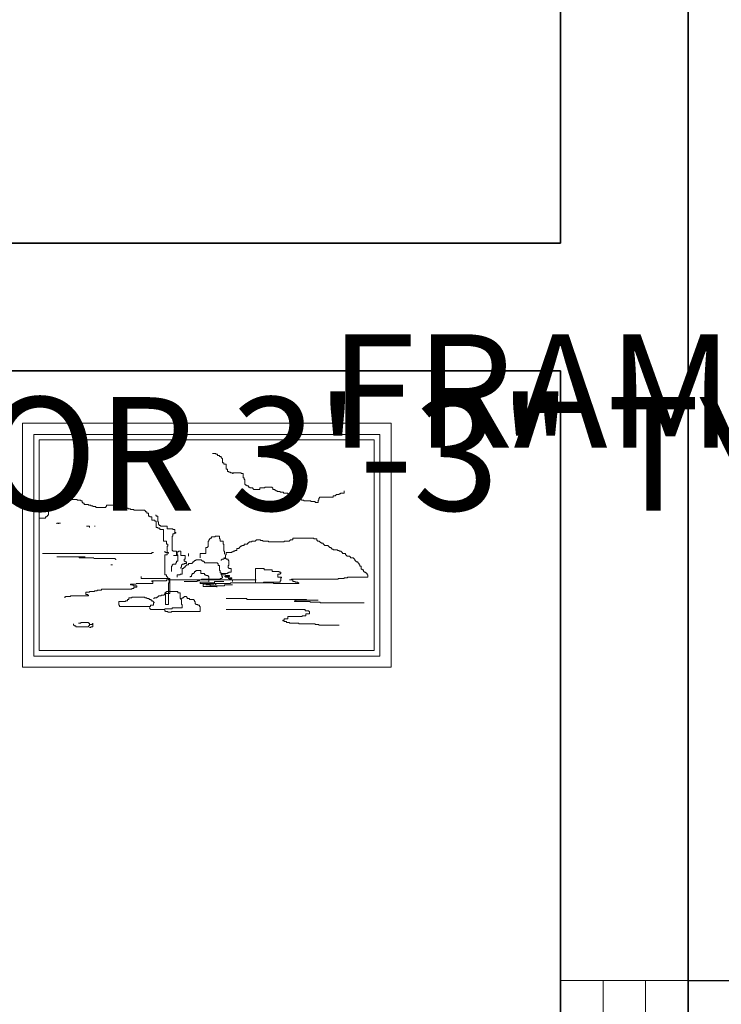
# Model space of a CAD drawing. Units: inches. Extents: x 125 to 976, y 231 to 853.
# Tile 7 of 16: x 418 to 468, y 449 to 519. Entities that reach past the tile are written whole.
import ezdxf

# ---------------------------------------------------------------- set-up
doc = ezdxf.new("R2010")
doc.units = ezdxf.units.IN
doc.header["$MEASUREMENT"] = 0
for name, color, linetype, lineweight in [('A-ANNO-DIMS', 2, 'Continuous', 18), ('A-FURN-ARTW', 9, 'Continuous', 13), ('A-GLAZ', 4, 'Continuous', 18), ('A-WALL', 7, 'Continuous', 35)]:
    doc.layers.add(name, color=color, linetype=linetype, lineweight=lineweight)
doc.styles.get("Standard").update_dxf_attribs({"font": 'italic8.shx'})
doc.dimstyles.get("Standard").update_dxf_attribs({"dimtxt": 8, "dimasz": 0.18, "dimexe": 0.18, "dimexo": 0.0625, "dimgap": 0.09, "dimtad": 0, "dimtih": 1, "dimtoh": 1, "dimdec": 4, "dimzin": 0, "dimdsep": 46, "dimlunit": 3, "dimtxsty": 'Standard', "dimcen": 0.09, "dimclrt": 4, "dimadec": 0, "dimazin": 0, "dimtfac": 1, "dimtdec": 4, "dimtofl": 0, "dimtmove": 0, "dimatfit": 3, "dimfxl": 1, "dimtolj": 1, "dimtzin": 0, "dimarcsym": 0})

# ---------------------------------------------------------------- blocks, each defined once
blk = doc.blocks.new('WINDOW-48IN')
for p, q in [((0.003, 0.005), (0.003, 48.005)), ((0.003, 48.005), (9.003, 48.005)), ((3.003, 0.005), (3.003, 48.005)), ((6.003, 0.005), (6.003, 48.005)), ((9.003, 48.005), (9.003, 0.005)), ((9.003, 0.005), (0.003, 0.005))]:
    blk.add_line(p, q)
blk = doc.blocks.new('*D40')
at = {"layer": 'A-ANNO-DIMS', "color": 0, "lineweight": -2, "transparency": 16777216}
for p, q in [((322.587, 494.042), (322.587, 488.075)), ((361.587, 494.042), (361.587, 488.075)), ((322.767, 488.255), (361.407, 488.255)), ((361.587, 488.255), (361.767, 488.255))]:
    blk.add_line(p, q, dxfattribs=at)
at = {"layer": 'A-ANNO-DIMS', "color": 0, "transparency": 16777216}
for points in [[(322.767, 488.285), (322.767, 488.225), (322.587, 488.255)], [(361.407, 488.285), (361.407, 488.225), (361.587, 488.255)]]:
    blk.add_solid(points, dxfattribs=at)
at = {"layer": 'Defpoints', "color": 0, "transparency": 16777216}
for p in [(322.587, 494.105), (361.587, 494.105), (361.587, 488.255)]:
    blk.add_point(p, dxfattribs=at)
at = {"layer": 'A-ANNO-DIMS', "color": 4, "transparency": 16777216, "insert": (432.523, 488.255), "char_height": 8, "attachment_point": 5}
blk.add_mtext('\\A1;RH DOOR 3\'-3" TYP.', dxfattribs=at)
blk = doc.blocks.new('*D44')
at = {"layer": 'A-ANNO-DIMS', "color": 0, "lineweight": -2, "transparency": 16777216}
for p, q in [((394.866, 489.715), (394.866, 492.869)), ((395.046, 492.689), (414.927, 492.689)), ((415.107, 489.715), (415.107, 492.869)), ((415.107, 492.689), (415.287, 492.689))]:
    blk.add_line(p, q, dxfattribs=at)
at = {"layer": 'A-ANNO-DIMS', "color": 0, "transparency": 16777216}
for points in [[(395.046, 492.719), (395.046, 492.659), (394.866, 492.689)], [(414.927, 492.719), (414.927, 492.659), (415.107, 492.689)]]:
    blk.add_solid(points, dxfattribs=at)
at = {"layer": 'Defpoints', "color": 0, "transparency": 16777216}
for p in [(415.107, 492.689), (394.866, 489.652), (415.107, 489.652)]:
    blk.add_point(p, dxfattribs=at)
at = {"layer": 'A-ANNO-DIMS', "color": 4, "transparency": 16777216, "insert": (498.425, 492.689), "char_height": 8, "attachment_point": 5}
blk.add_mtext('\\A1;FRAMED ART 1\'-8" TYP.', dxfattribs=at)
blk = doc.blocks.new('*D64')
at = {"layer": 'A-ANNO-DIMS', "color": 0, "lineweight": -2, "transparency": 16777216}
for p, q in [((465.642, 658.828), (494.459, 658.828)), ((494.279, 658.648), (494.279, 561.162)), ((494.279, 451.305), (494.279, 548.792)), ((465.642, 451.125), (494.459, 451.125))]:
    blk.add_line(p, q, dxfattribs=at)
at = {"layer": 'A-ANNO-DIMS', "color": 0, "transparency": 16777216}
for points in [[(494.249, 658.648), (494.309, 658.648), (494.279, 658.828)], [(494.249, 451.305), (494.309, 451.305), (494.279, 451.125)]]:
    blk.add_solid(points, dxfattribs=at)
at = {"layer": 'Defpoints', "color": 0, "transparency": 16777216}
for p in [(465.579, 658.828), (494.279, 658.828), (465.579, 451.125)]:
    blk.add_point(p, dxfattribs=at)
at = {"layer": 'A-ANNO-DIMS', "color": 4, "transparency": 16777216, "insert": (494.279, 554.977), "char_height": 8, "attachment_point": 5}
blk.add_mtext('\\A1;17\'-3 1/2"', dxfattribs=at)

msp = doc.modelspace()

# ---------------------------------------------------------------- linework, layer by layer
at = {"layer": 'A-FURN-ARTW'}
for p, q in [((418.65967, 490.41771), (418.65967, 473.20521)), ((444.63356, 490.41771), (418.65967, 490.41771)), ((444.63356, 473.20521), (444.63356, 490.41771)), ((432.04117, 488.28145), (432.29476, 488.28145)), ((432.29476, 488.28145), (432.29476, 488.23077)), ((432.29476, 488.23077), (432.3962, 488.23077)), ((432.3962, 488.23077), (432.3962, 488.1294)), ((432.3962, 488.1294), (432.54835, 488.1294)), ((432.54835, 488.1294), (432.54835, 488.07871)), ((432.54835, 488.07871), (432.64979, 488.07871)), ((432.64979, 488.07871), (432.64979, 487.97734)), ((432.64979, 487.97734), (432.70051, 487.97734)), ((432.70051, 487.97734), (432.70051, 487.92666)), ((432.70051, 487.92666), (432.75123, 487.92666)), ((432.75123, 487.92666), (432.75123, 487.62255)), ((432.75123, 487.62255), (432.85267, 487.62255)), ((432.85267, 487.62255), (432.85267, 487.52118)), ((432.85267, 487.52118), (433.00482, 487.52118)), ((433.00482, 487.52118), (433.00482, 487.16639)), ((433.00482, 487.16639), (433.10626, 487.16639)), ((433.10626, 487.16639), (433.10626, 487.01434)), ((433.10626, 487.01434), (433.2077, 487.01434)), ((433.2077, 487.01434), (433.2077, 486.96365)), ((433.2077, 486.96365), (433.30913, 486.96365)), ((433.30913, 486.96365), (433.30913, 486.91297)), ((433.30913, 486.91297), (433.46129, 486.91297)), ((433.46129, 486.91297), (433.46129, 486.86228)), ((433.46129, 486.86228), (433.51201, 486.86228)), ((433.51201, 486.86228), (433.51201, 486.91297)), ((433.51201, 486.91297), (434.06991, 486.91297)), ((434.06991, 486.91297), (434.06991, 486.86228)), ((434.06991, 486.86228), (434.22207, 486.86228)), ((434.22207, 486.86228), (434.22207, 486.55818)), ((434.22207, 486.55818), (434.27279, 486.55818)), ((434.27279, 486.55818), (434.27279, 486.45681)), ((434.27279, 486.45681), (434.32351, 486.45681)), ((434.32351, 486.45681), (434.32351, 486.10202)), ((434.32351, 486.10202), (434.37423, 486.10202)), ((434.37423, 486.10202), (434.37423, 486.05133)), ((434.37423, 486.05133), (434.47566, 486.05133)), ((434.47566, 486.05133), (434.47566, 486.00065)), ((434.47566, 486.00065), (434.5771, 486.00065)), ((434.5771, 486.00065), (434.5771, 485.89928)), ((434.5771, 485.89928), (434.67854, 485.89928)), ((434.67854, 485.89928), (434.67854, 485.8486)), ((434.67854, 485.8486), (434.88141, 485.8486)), ((434.88141, 485.8486), (434.88141, 485.79791)), ((434.88141, 485.79791), (434.93213, 485.79791)), ((434.93213, 485.79791), (434.93213, 485.74723)), ((434.93213, 485.74723), (435.3886, 485.74723)), ((435.3886, 485.74723), (435.3886, 485.8486)), ((435.3886, 485.8486), (435.74363, 485.8486)), ((435.74363, 485.8486), (435.74363, 485.89928)), ((435.74363, 485.89928), (436.25082, 485.89928)), ((436.25082, 485.89928), (436.25082, 485.8486)), ((436.25082, 485.8486), (436.30153, 485.8486)), ((436.30153, 485.8486), (436.30153, 485.74723)), ((436.30153, 485.74723), (436.45369, 485.74723)), ((436.45369, 485.74723), (436.45369, 485.69654)), ((436.45369, 485.69654), (436.50441, 485.69654)), ((436.50441, 485.69654), (436.50441, 485.64586)), ((436.50441, 485.64586), (436.60585, 485.64586)), ((436.60585, 485.64586), (436.60585, 485.59517)), ((436.60585, 485.59517), (436.80872, 485.59517)), ((436.80872, 485.59517), (436.80872, 485.54449)), ((436.80872, 485.54449), (437.06231, 485.54449)), ((437.06231, 485.54449), (437.06231, 485.49381)), ((437.06231, 485.49381), (437.36663, 485.49381)), ((437.36663, 485.49381), (437.36663, 485.44312)), ((437.36663, 485.44312), (437.5695, 485.44312)), ((437.5695, 485.44312), (437.5695, 485.39244)), ((437.5695, 485.39244), (437.62022, 485.39244)), ((437.62022, 485.39244), (437.62022, 485.13901)), ((440.76478, 485.34175), (440.76478, 485.39244)), ((440.76478, 485.39244), (440.96765, 485.39244)), ((440.96765, 485.39244), (440.96765, 485.44312)), ((440.96765, 485.44312), (441.06909, 485.44312)), ((441.06909, 485.44312), (441.06909, 485.49381)), ((441.06909, 485.49381), (441.32268, 485.49381)), ((441.32268, 485.49381), (441.32268, 485.64586)), ((421.13666, 484.63217), (421.13666, 484.68285)), ((421.13666, 484.68285), (421.23809, 484.68285)), ((421.23809, 484.68285), (421.23809, 484.88559)), ((421.23809, 484.88559), (421.28881, 484.88559)), ((421.28881, 484.88559), (421.28881, 484.93628)), ((421.28881, 484.93628), (421.5424, 484.93628)), ((421.5424, 484.93628), (421.5424, 484.98696)), ((421.5424, 484.98696), (421.74528, 484.98696)), ((421.74528, 484.98696), (421.74528, 485.03765)), ((421.74528, 485.03765), (422.50606, 485.03765)), ((422.50606, 485.03765), (422.50606, 484.98696)), ((422.50606, 484.98696), (422.75965, 484.98696)), ((422.75965, 484.98696), (422.75965, 484.93628)), ((422.75965, 484.93628), (422.86109, 484.93628)), ((422.86109, 484.93628), (422.86109, 484.83491)), ((422.86109, 484.83491), (422.91181, 484.83491)), ((422.91181, 484.83491), (422.91181, 484.78422)), ((422.91181, 484.78422), (423.01325, 484.78422)), ((423.01325, 484.78422), (423.01325, 484.68285)), ((423.01325, 484.68285), (423.31756, 484.68285)), ((423.31756, 484.68285), (423.31756, 484.63217)), ((437.62022, 485.13901), (437.72166, 485.13901)), ((437.72166, 485.13901), (437.72166, 485.08833)), ((437.72166, 485.08833), (438.12741, 485.08833)), ((438.12741, 485.08833), (438.12741, 485.03765)), ((438.12741, 485.03765), (438.33028, 485.03765)), ((438.33028, 485.03765), (438.33028, 484.98696)), ((438.33028, 484.98696), (438.48244, 484.98696)), ((438.48244, 484.98696), (438.48244, 484.93628)), ((438.48244, 484.93628), (438.98962, 484.93628)), ((438.98962, 484.93628), (438.98962, 484.88559)), ((438.98962, 484.88559), (439.29394, 484.88559)), ((439.29394, 484.88559), (439.29394, 484.83491)), ((439.29394, 484.83491), (439.49681, 484.83491)), ((439.49681, 484.83491), (439.49681, 484.98696)), ((439.49681, 484.98696), (439.54753, 484.98696)), ((439.54753, 484.98696), (439.54753, 485.13901)), ((439.54753, 485.13901), (439.59825, 485.13901)), ((439.59825, 485.13901), (439.59825, 485.1897)), ((439.59825, 485.1897), (440.5619, 485.1897)), ((440.5619, 485.1897), (440.5619, 485.29107)), ((440.5619, 485.29107), (440.71406, 485.29107)), ((440.71406, 485.29107), (440.71406, 485.34175)), ((440.71406, 485.34175), (440.76478, 485.34175)), ((420.47731, 483.92259), (420.47731, 484.37875)), ((420.47731, 484.37875), (420.88306, 484.37875)), ((420.88306, 484.37875), (420.88306, 484.42943)), ((420.88306, 484.42943), (420.93378, 484.42943)), ((420.93378, 484.42943), (420.93378, 484.48012)), ((420.93378, 484.48012), (420.9845, 484.48012)), ((420.9845, 484.48012), (420.9845, 484.58149)), ((420.9845, 484.58149), (421.03522, 484.58149)), ((421.03522, 484.58149), (421.03522, 484.63217)), ((421.03522, 484.63217), (421.13666, 484.63217)), ((423.31756, 484.63217), (423.46971, 484.63217)), ((423.46971, 484.63217), (423.46971, 484.58149)), ((423.46971, 484.58149), (423.62187, 484.58149)), ((423.62187, 484.58149), (423.62187, 484.5308)), ((423.62187, 484.5308), (423.82474, 484.5308)), ((423.82474, 484.5308), (423.82474, 484.48012)), ((423.82474, 484.48012), (424.53481, 484.48012)), ((424.53481, 484.48012), (424.53481, 484.5308)), ((424.53481, 484.5308), (424.58552, 484.5308)), ((424.58552, 484.5308), (424.58552, 484.63217)), ((424.58552, 484.63217), (425.29559, 484.63217)), ((425.29559, 484.63217), (425.29559, 484.58149)), ((425.29559, 484.58149), (425.44774, 484.58149)), ((425.44774, 484.58149), (425.44774, 484.5308)), ((425.44774, 484.5308), (425.54918, 484.5308)), ((425.54918, 484.5308), (425.54918, 484.48012)), ((425.54918, 484.48012), (426.00565, 484.48012)), ((426.00565, 484.48012), (426.00565, 484.42943)), ((426.00565, 484.42943), (426.10708, 484.42943)), ((426.10708, 484.42943), (426.10708, 484.37875)), ((426.10708, 484.37875), (426.25924, 484.37875)), ((426.25924, 484.37875), (426.25924, 484.32806)), ((426.25924, 484.32806), (426.51283, 484.32806)), ((426.51283, 484.32806), (426.51283, 484.27738)), ((426.51283, 484.27738), (427.27361, 484.27738)), ((427.27361, 484.27738), (427.27361, 484.22669)), ((427.27361, 484.22669), (427.32433, 484.22669)), ((427.32433, 484.22669), (427.32433, 484.17601)), ((427.32433, 484.17601), (427.42577, 484.17601)), ((427.42577, 484.17601), (427.42577, 484.07464)), ((427.42577, 484.07464), (427.52721, 484.07464)), ((427.52721, 484.07464), (427.52721, 483.8719)), ((419.86869, 483.71985), (420.27444, 483.71985)), ((420.27444, 483.71985), (420.27444, 483.82122)), ((420.27444, 483.82122), (420.37588, 483.82122)), ((420.37588, 483.82122), (420.37588, 483.8719)), ((420.37588, 483.8719), (420.4266, 483.8719)), ((420.4266, 483.8719), (420.4266, 483.92259)), ((420.4266, 483.92259), (420.47731, 483.92259)), ((421.08594, 483.31437), (421.08594, 483.36506)), ((421.08594, 483.36506), (421.18738, 483.36506)), ((421.18738, 483.36506), (421.18738, 483.31437)), ((421.18738, 483.31437), (421.18738, 483.36506)), ((421.18738, 483.36506), (421.33953, 483.36506)), ((427.52721, 483.8719), (427.62864, 483.8719)), ((427.62864, 483.8719), (427.62864, 483.82122)), ((427.62864, 483.82122), (427.7808, 483.82122)), ((427.7808, 483.82122), (427.7808, 483.5678)), ((427.7808, 483.5678), (427.98368, 483.5678)), ((427.98368, 483.5678), (427.98368, 483.51711)), ((427.98368, 483.51711), (428.08511, 483.51711)), ((428.03439, 483.92259), (428.08511, 483.92259)), ((428.08511, 483.92259), (428.08511, 483.8719)), ((428.08511, 483.8719), (428.18655, 483.8719)), ((428.08511, 483.51711), (428.08511, 483.06095)), ((428.18655, 483.8719), (428.18655, 483.46643)), ((428.18655, 483.46643), (428.23727, 483.46643)), ((428.23727, 483.46643), (428.23727, 483.26369)), ((423.1654, 483.16232), (423.36828, 483.16232)), ((423.36828, 483.16232), (423.36828, 483.06095)), ((423.72331, 483.16232), (423.77403, 483.16232)), ((428.08511, 483.06095), (428.18655, 483.06095)), ((428.18655, 483.06095), (428.18655, 483.01027)), ((428.18655, 483.01027), (428.33871, 483.01027)), ((428.23727, 483.26369), (428.28799, 483.26369)), ((428.28799, 483.26369), (428.28799, 483.213)), ((428.28799, 483.213), (428.38942, 483.213)), ((428.33871, 483.01027), (428.33871, 482.9089)), ((428.33871, 482.9089), (428.5923, 482.9089)), ((428.38942, 483.213), (428.38942, 483.16232)), ((428.38942, 483.16232), (428.84589, 483.16232)), ((428.5923, 482.9089), (428.5923, 482.09795)), ((428.84589, 483.16232), (428.84589, 482.95958)), ((428.84589, 482.95958), (429.25164, 482.95958)), ((429.25164, 482.95958), (429.25164, 482.9089)), ((429.25164, 482.9089), (429.4038, 482.9089)), ((429.35308, 482.60479), (429.25164, 482.60479)), ((429.25164, 482.60479), (429.25164, 482.45274)), ((429.45452, 482.65547), (429.35308, 482.65547)), ((429.35308, 482.65547), (429.35308, 482.60479)), ((429.4038, 482.9089), (429.4038, 482.70616)), ((429.4038, 482.70616), (429.45452, 482.70616)), ((429.45452, 482.70616), (429.45452, 482.65547)), ((428.5923, 482.09795), (428.79517, 482.09795)), ((428.79517, 482.09795), (428.79517, 481.89521)), ((429.25164, 482.45274), (429.20092, 482.45274)), ((429.20092, 482.45274), (429.20092, 481.43905)), ((431.73686, 481.69247), (431.73686, 482.09795)), ((431.73686, 482.09795), (431.78757, 482.09795)), ((431.78757, 482.09795), (431.78757, 482.19932)), ((431.78757, 482.19932), (431.83829, 482.19932)), ((431.83829, 482.19932), (431.83829, 482.25)), ((431.83829, 482.25), (431.88901, 482.25)), ((431.88901, 482.25), (431.88901, 482.30068)), ((431.88901, 482.30068), (431.99045, 482.30068)), ((431.99045, 482.30068), (431.99045, 482.40205)), ((431.99045, 482.40205), (432.24404, 482.40205)), ((432.24404, 482.40205), (432.24404, 482.45274)), ((432.24404, 482.45274), (432.54835, 482.45274)), ((432.54835, 482.45274), (432.54835, 482.25)), ((432.54835, 482.25), (432.59907, 482.25)), ((432.59907, 482.25), (432.59907, 482.09795)), ((432.59907, 482.09795), (432.80195, 482.09795)), ((432.80195, 482.09795), (432.80195, 481.89521)), ((434.52638, 481.89521), (434.52638, 481.94589)), ((434.52638, 481.94589), (434.5771, 481.94589)), ((434.5771, 481.94589), (434.5771, 481.99658)), ((434.5771, 481.99658), (434.62782, 481.99658)), ((434.62782, 481.99658), (434.62782, 482.04726)), ((434.62782, 482.04726), (434.83069, 482.04726)), ((434.83069, 482.04726), (434.83069, 482.09795)), ((434.83069, 482.09795), (435.08429, 482.09795)), ((435.08429, 482.09795), (435.08429, 482.14863)), ((435.08429, 482.14863), (435.13501, 482.14863)), ((435.13501, 482.14863), (435.13501, 482.19932)), ((435.13501, 482.19932), (435.43932, 482.19932)), ((435.43932, 482.19932), (435.43932, 482.14863)), ((435.43932, 482.14863), (435.59147, 482.14863)), ((435.59147, 482.14863), (435.59147, 482.09795)), ((435.59147, 482.09795), (435.99722, 482.09795)), ((435.99722, 482.09795), (435.99722, 482.04726)), ((435.99722, 482.04726), (437.11303, 482.04726)), ((437.11303, 482.04726), (437.11303, 482.09795)), ((437.11303, 482.09795), (437.46806, 482.09795)), ((437.46806, 482.09795), (437.46806, 482.14863)), ((437.46806, 482.14863), (437.51878, 482.14863)), ((437.51878, 482.14863), (437.51878, 482.19932)), ((437.51878, 482.19932), (437.72166, 482.19932)), ((437.72166, 482.30068), (439.1925, 482.30068)), ((437.72166, 482.19932), (437.72166, 482.30068)), ((439.1925, 482.30068), (439.1925, 482.25)), ((439.1925, 482.25), (439.39537, 482.25)), ((439.39537, 482.25), (439.39537, 482.14863)), ((439.39537, 482.14863), (439.44609, 482.14863)), ((439.44609, 482.14863), (439.44609, 482.09795)), ((439.44609, 482.09795), (439.59825, 482.09795)), ((439.59825, 482.09795), (439.59825, 482.04726)), ((439.59825, 482.04726), (439.64897, 482.04726)), ((439.64897, 482.04726), (439.64897, 481.99658)), ((439.64897, 481.99658), (439.69968, 481.99658)), ((439.69968, 481.99658), (439.69968, 481.94589)), ((439.69968, 481.94589), (439.85184, 481.94589)), ((439.85184, 481.94589), (439.85184, 481.89521)), ((420.07157, 481.23631), (427.7808, 481.23631)), ((427.7808, 481.23631), (427.7808, 481.287)), ((427.7808, 481.287), (427.88224, 481.287)), ((428.64302, 481.33768), (428.74445, 481.33768)), ((428.74445, 481.33768), (428.74445, 481.287)), ((428.74445, 481.287), (428.94733, 481.287)), ((428.79517, 481.89521), (428.89661, 481.89521)), ((428.89661, 481.74316), (428.84589, 481.74316)), ((428.84589, 481.74316), (428.84589, 481.13494)), ((428.89661, 481.89521), (428.89661, 481.74316)), ((428.94733, 481.287), (428.94733, 481.23631)), ((429.20092, 481.43905), (429.25164, 481.43905)), ((429.25164, 481.43905), (429.25164, 481.38837)), ((429.25164, 481.38837), (429.50523, 481.38837)), ((429.50523, 481.38837), (429.50523, 481.13494)), ((429.55595, 481.08426), (429.55595, 481.33768)), ((429.55595, 481.33768), (429.65739, 481.33768)), ((429.65739, 481.33768), (429.65739, 481.38837)), ((429.65739, 481.38837), (429.80955, 481.38837)), ((429.80955, 481.38837), (429.80955, 481.08426)), ((430.36745, 481.23631), (430.36745, 481.03357)), ((431.17895, 480.93221), (431.17895, 481.23631)), ((431.17895, 481.23631), (431.5847, 481.23631)), ((431.5847, 481.23631), (431.5847, 481.64179)), ((431.5847, 481.64179), (431.68614, 481.64179)), ((431.68614, 481.64179), (431.68614, 481.69247)), ((431.68614, 481.69247), (431.73686, 481.69247)), ((432.80195, 481.89521), (432.85267, 481.89521)), ((432.85267, 481.89521), (432.85267, 481.38837)), ((432.85267, 481.38837), (432.90339, 481.38837)), ((432.90339, 481.38837), (432.90339, 481.18563)), ((433.00482, 481.13494), (433.00482, 481.287)), ((433.00482, 481.287), (433.41057, 481.287)), ((433.41057, 481.287), (433.41057, 481.33768)), ((433.41057, 481.33768), (433.51201, 481.33768)), ((433.51201, 481.33768), (433.51201, 481.38837)), ((433.51201, 481.38837), (433.61345, 481.38837)), ((433.61345, 481.38837), (433.61345, 481.43905)), ((433.61345, 481.43905), (433.7656, 481.43905)), ((433.7656, 481.43905), (433.7656, 481.5911)), ((433.7656, 481.5911), (433.91776, 481.5911)), ((433.91776, 481.5911), (433.91776, 481.64179)), ((433.91776, 481.64179), (433.96848, 481.64179)), ((433.96848, 481.64179), (433.96848, 481.69247)), ((433.96848, 481.69247), (434.01919, 481.69247)), ((434.01919, 481.69247), (434.01919, 481.74316)), ((434.01919, 481.74316), (434.12063, 481.74316)), ((434.12063, 481.74316), (434.12063, 481.79384)), ((434.12063, 481.79384), (434.27279, 481.79384)), ((434.27279, 481.79384), (434.27279, 481.89521)), ((434.27279, 481.89521), (434.52638, 481.89521)), ((439.85184, 481.89521), (439.90256, 481.89521)), ((439.90256, 481.89521), (439.90256, 481.84452)), ((439.90256, 481.84452), (439.95328, 481.84452)), ((439.95328, 481.84452), (439.95328, 481.79384)), ((439.95328, 481.79384), (440.20687, 481.79384)), ((440.20687, 481.79384), (440.20687, 481.74316)), ((440.20687, 481.74316), (440.25759, 481.74316)), ((440.25759, 481.74316), (440.25759, 481.69247)), ((440.25759, 481.69247), (440.30831, 481.69247)), ((440.30831, 481.69247), (440.30831, 481.64179)), ((440.30831, 481.64179), (440.40975, 481.64179)), ((440.40975, 481.64179), (440.40975, 481.5911)), ((440.40975, 481.5911), (440.46046, 481.5911)), ((440.46046, 481.5911), (440.46046, 481.54042)), ((440.46046, 481.54042), (440.5619, 481.54042)), ((440.5619, 481.54042), (440.5619, 481.48973)), ((440.5619, 481.48973), (440.86621, 481.48973)), ((440.86621, 481.48973), (440.86621, 481.43905)), ((440.86621, 481.43905), (440.96765, 481.43905)), ((440.96765, 481.43905), (440.96765, 481.38837)), ((440.96765, 481.38837), (441.11981, 481.38837)), ((441.11981, 481.38837), (441.11981, 481.33768)), ((441.11981, 481.33768), (441.17053, 481.33768)), ((441.17053, 481.33768), (441.17053, 481.287)), ((441.17053, 481.287), (441.22124, 481.287)), ((441.22124, 481.287), (441.22124, 481.23631)), ((441.22124, 481.23631), (441.42412, 481.23631)), ((441.42412, 481.23631), (441.42412, 481.13494)), ((421.08594, 480.98289), (423.06396, 480.98289)), ((423.06396, 480.98289), (422.6075, 480.98289)), ((422.6075, 480.98289), (422.65822, 480.98289)), ((422.65822, 480.98289), (422.65822, 480.93221)), ((422.65822, 480.93221), (423.67259, 480.93221)), ((423.67259, 480.88152), (425.19415, 480.88152)), ((425.19415, 480.88152), (425.19415, 480.83084)), ((425.19415, 480.83084), (425.24487, 480.83084)), ((425.24487, 480.83084), (425.24487, 480.78015)), ((428.84589, 481.13494), (428.69374, 481.13494)), ((428.69374, 481.13494), (428.69374, 479.71578)), ((429.30236, 481.08426), (429.55595, 481.08426)), ((429.50523, 480.57741), (429.45452, 480.57741)), ((429.45452, 480.57741), (429.45452, 480.47604)), ((429.50523, 481.13494), (429.60667, 481.13494)), ((429.60667, 480.67878), (429.50523, 480.67878)), ((429.50523, 480.67878), (429.50523, 480.57741)), ((429.60667, 481.13494), (429.60667, 480.67878)), ((429.80955, 481.08426), (430.11386, 481.08426)), ((430.11386, 480.83084), (430.06314, 480.83084)), ((430.06314, 480.83084), (430.06314, 480.67878)), ((430.06314, 480.67878), (430.11386, 480.67878)), ((430.2153, 480.52673), (430.06314, 480.52673)), ((430.06314, 480.52673), (430.06314, 480.47604)), ((430.11386, 481.08426), (430.11386, 480.83084)), ((430.11386, 480.67878), (430.11386, 480.6281)), ((430.11386, 480.6281), (430.2153, 480.6281)), ((430.2153, 480.6281), (430.2153, 480.52673)), ((430.36745, 480.42536), (430.36745, 480.52673)), ((430.36745, 480.52673), (430.62105, 480.52673)), ((430.62105, 480.52673), (430.62105, 480.57741)), ((430.62105, 480.57741), (430.67176, 480.57741)), ((430.67176, 480.57741), (430.67176, 480.6281)), ((430.67176, 480.6281), (430.72248, 480.6281)), ((430.72248, 480.6281), (430.72248, 480.67878)), ((430.72248, 480.67878), (430.7732, 480.67878)), ((430.7732, 480.67878), (430.7732, 480.72947)), ((430.7732, 480.72947), (430.87464, 480.72947)), ((430.87464, 480.72947), (430.87464, 480.78015)), ((430.87464, 480.78015), (431.28039, 480.78015)), ((431.28039, 480.78015), (431.28039, 480.72947)), ((431.28039, 480.72947), (431.33111, 480.72947)), ((431.33111, 480.72947), (431.33111, 480.67878)), ((431.33111, 480.67878), (431.43254, 480.67878)), ((431.43254, 480.67878), (431.43254, 480.6281)), ((431.43254, 480.6281), (431.48326, 480.6281)), ((431.48326, 480.6281), (431.48326, 480.57741)), ((431.48326, 480.57741), (432.3962, 480.57741)), ((432.3962, 480.57741), (432.3962, 480.52673)), ((432.3962, 480.52673), (432.44692, 480.52673)), ((432.44692, 480.52673), (432.44692, 480.37468)), ((432.64979, 480.72947), (432.64979, 480.78015)), ((432.64979, 480.78015), (432.70051, 480.78015)), ((432.70051, 480.78015), (432.70051, 480.83084)), ((432.70051, 480.83084), (432.85267, 480.83084)), ((432.85267, 480.93221), (432.90339, 480.93221)), ((432.85267, 480.83084), (432.85267, 480.88152)), ((432.85267, 480.88152), (432.9541, 480.88152)), ((432.90339, 480.93221), (432.90339, 480.88152)), ((432.90339, 480.88152), (433.00482, 480.88152)), ((432.9541, 480.88152), (432.9541, 481.13494)), ((432.9541, 481.13494), (433.00482, 481.13494)), ((433.00482, 480.88152), (433.00482, 480.83084)), ((433.00482, 480.83084), (433.15698, 480.83084)), ((433.15698, 480.83084), (433.15698, 480.72947)), ((433.15698, 480.72947), (433.2077, 480.72947)), ((433.2077, 480.72947), (433.2077, 480.37468)), ((441.42412, 481.13494), (441.47484, 481.13494)), ((441.47484, 481.13494), (441.47484, 481.08426)), ((441.47484, 481.08426), (441.52556, 481.08426)), ((441.52556, 481.08426), (441.52556, 481.03357)), ((441.52556, 481.03357), (441.72843, 481.03357)), ((441.72843, 481.03357), (441.72843, 480.98289)), ((441.72843, 480.98289), (441.77915, 480.98289)), ((441.77915, 480.98289), (441.77915, 480.93221)), ((441.77915, 480.93221), (441.98202, 480.93221)), ((441.98202, 480.93221), (441.98202, 480.88152)), ((441.98202, 480.88152), (442.03274, 480.88152)), ((442.03274, 480.88152), (442.03274, 480.83084)), ((442.03274, 480.83084), (442.08346, 480.83084)), ((442.08346, 480.83084), (442.08346, 480.72947)), ((442.08346, 480.72947), (442.13418, 480.72947)), ((442.13418, 480.72947), (442.13418, 480.67878)), ((442.13418, 480.67878), (442.1849, 480.67878)), ((442.1849, 480.67878), (442.1849, 480.6281)), ((442.1849, 480.6281), (442.28634, 480.6281)), ((442.28634, 480.6281), (442.28634, 480.57741)), ((442.28634, 480.57741), (442.33706, 480.57741)), ((442.33706, 480.57741), (442.33706, 480.52673)), ((442.33706, 480.52673), (442.38777, 480.52673)), ((442.38777, 480.52673), (442.38777, 480.42536)), ((424.99127, 480.42536), (424.88984, 480.42536)), ((429.20092, 480.32399), (429.1502, 480.32399)), ((429.1502, 480.32399), (429.1502, 479.9692)), ((429.25164, 480.42536), (429.20092, 480.42536)), ((429.20092, 480.42536), (429.20092, 480.32399)), ((429.45452, 480.47604), (429.25164, 480.47604)), ((429.25164, 480.47604), (429.25164, 480.42536)), ((429.86027, 480.27331), (429.80955, 480.27331)), ((429.80955, 480.27331), (429.80955, 480.17194)), ((429.91098, 480.42536), (429.86027, 480.42536)), ((429.86027, 480.42536), (429.86027, 480.27331)), ((430.06314, 480.47604), (429.91098, 480.47604)), ((429.91098, 480.47604), (429.91098, 480.42536)), ((429.91098, 479.76646), (429.91098, 480.17194)), ((429.91098, 480.17194), (430.01242, 480.17194)), ((430.01242, 480.17194), (430.01242, 480.22262)), ((430.01242, 480.22262), (430.06314, 480.22262)), ((430.06314, 480.22262), (430.06314, 480.27331)), ((430.06314, 480.27331), (430.11386, 480.27331)), ((430.11386, 480.27331), (430.11386, 480.32399)), ((430.11386, 480.32399), (430.16458, 480.32399)), ((430.16458, 480.32399), (430.16458, 480.37468)), ((430.16458, 480.37468), (430.2153, 480.37468)), ((430.2153, 480.37468), (430.2153, 480.42536)), ((430.2153, 480.42536), (430.36745, 480.42536)), ((430.72248, 479.81715), (430.72248, 479.86783)), ((430.72248, 479.86783), (430.7732, 479.86783)), ((430.7732, 479.86783), (430.7732, 479.9692)), ((430.7732, 479.9692), (430.87464, 479.9692)), ((430.87464, 479.9692), (430.87464, 480.01988)), ((430.87464, 480.01988), (431.22967, 480.01988)), ((431.22967, 480.01988), (431.22967, 479.81715)), ((432.44692, 480.37468), (432.54835, 480.37468)), ((432.54835, 480.37468), (432.54835, 480.01988)), ((432.54835, 480.01988), (432.59907, 480.01988)), ((432.59907, 480.01988), (432.59907, 479.86783)), ((432.59907, 479.86783), (432.64979, 479.86783)), ((432.64979, 479.86783), (432.64979, 479.81715)), ((433.2077, 479.86783), (433.10626, 479.86783)), ((433.10626, 479.86783), (433.10626, 479.81715)), ((433.2077, 480.37468), (433.15698, 480.37468)), ((433.15698, 480.37468), (433.15698, 480.22262)), ((433.15698, 480.22262), (433.2077, 480.22262)), ((433.2077, 480.22262), (433.2077, 480.17194)), ((433.2077, 480.17194), (433.35985, 480.17194)), ((433.35985, 479.91852), (433.2077, 479.91852)), ((433.2077, 479.91852), (433.2077, 479.86783)), ((433.35985, 480.17194), (433.35985, 479.91852)), ((435.69291, 480.17194), (435.08429, 480.17194)), ((435.08429, 480.17194), (435.08429, 479.20893)), ((435.69291, 480.07057), (435.69291, 480.17194)), ((436.25082, 480.07057), (435.69291, 480.07057)), ((436.25082, 479.9692), (436.25082, 480.07057)), ((436.758, 479.9692), (436.25082, 479.9692)), ((436.758, 479.91852), (436.758, 479.9692)), ((436.85944, 479.91852), (436.758, 479.91852)), ((436.85944, 479.81715), (436.85944, 479.91852)), ((442.38777, 480.42536), (442.43849, 480.42536)), ((442.43849, 480.42536), (442.43849, 480.32399)), ((442.43849, 480.32399), (442.53993, 480.32399)), ((442.53993, 480.32399), (442.53993, 480.12125)), ((442.53993, 480.12125), (442.59065, 480.12125)), ((442.59065, 480.12125), (442.59065, 480.07057)), ((442.59065, 480.07057), (442.69209, 480.07057)), ((442.69209, 480.07057), (442.69209, 479.9692)), ((442.69209, 479.9692), (442.7428, 479.9692)), ((442.7428, 479.9692), (442.7428, 479.91852)), ((442.7428, 479.91852), (442.84424, 479.91852)), ((442.84424, 479.91852), (442.84424, 479.86783)), ((442.84424, 479.86783), (442.89496, 479.86783)), ((442.89496, 479.86783), (442.89496, 479.81715)), ((427.02002, 479.46236), (427.02002, 479.61441)), ((429.04877, 479.46236), (427.02002, 479.46236)), ((428.79517, 479.3103), (427.7808, 479.3103)), ((427.7808, 479.3103), (427.7808, 479.25962)), ((427.7808, 479.25962), (427.83152, 479.25962)), ((427.83152, 479.25962), (427.83152, 479.10756)), ((428.69374, 479.71578), (428.79517, 479.71578)), ((428.79517, 479.71578), (428.79517, 479.61441)), ((428.79517, 479.61441), (428.84589, 479.61441)), ((428.94733, 479.36099), (428.79517, 479.36099)), ((428.79517, 479.36099), (428.79517, 479.3103)), ((428.84589, 479.61441), (428.84589, 479.56372)), ((428.84589, 479.56372), (428.89661, 479.56372)), ((428.89661, 479.56372), (428.89661, 479.46236)), ((428.89661, 479.46236), (429.04877, 479.46236)), ((429.04877, 479.41167), (428.94733, 479.41167)), ((428.94733, 479.41167), (428.94733, 479.36099)), ((428.99805, 479.15825), (428.94733, 479.15825)), ((428.94733, 479.15825), (428.94733, 477.63772)), ((435.13501, 479.36099), (428.99805, 479.36099)), ((428.99805, 479.36099), (428.99805, 479.15825)), ((429.04877, 479.46236), (429.04877, 479.41167)), ((429.04877, 478.39798), (429.04877, 479.46236)), ((429.55595, 479.56372), (429.55595, 479.71578)), ((429.55595, 479.71578), (429.75883, 479.71578)), ((429.75883, 479.71578), (429.75883, 479.76646)), ((429.75883, 479.76646), (429.91098, 479.76646)), ((430.97608, 479.25962), (430.06314, 479.25962)), ((430.46889, 479.56372), (430.46889, 479.61441)), ((430.46889, 479.61441), (430.57033, 479.61441)), ((430.57033, 479.61441), (430.57033, 479.71578)), ((430.57033, 479.71578), (430.62105, 479.71578)), ((430.62105, 479.71578), (430.62105, 479.81715)), ((430.62105, 479.81715), (430.72248, 479.81715)), ((431.12823, 479.3103), (430.97608, 479.3103)), ((430.97608, 479.3103), (430.97608, 479.25962)), ((431.28039, 479.36099), (431.12823, 479.36099)), ((431.12823, 479.36099), (431.12823, 479.3103)), ((431.78757, 479.20893), (431.17895, 479.20893)), ((431.17895, 479.20893), (431.17895, 479.10756)), ((431.22967, 479.81715), (431.48326, 479.81715)), ((432.59907, 479.41167), (431.28039, 479.41167)), ((431.28039, 479.41167), (431.28039, 479.36099)), ((431.48326, 479.81715), (431.48326, 479.71578)), ((431.48326, 479.71578), (431.5847, 479.71578)), ((431.5847, 479.71578), (431.5847, 479.66509)), ((431.5847, 479.66509), (431.73686, 479.66509)), ((431.73686, 479.66509), (431.73686, 479.61441)), ((431.73686, 479.61441), (431.78757, 479.61441)), ((431.78757, 479.61441), (431.78757, 479.20893)), ((431.83829, 479.10756), (431.83829, 479.15825)), ((431.83829, 479.15825), (432.19332, 479.15825)), ((432.85267, 479.25962), (432.19332, 479.25962)), ((432.19332, 479.25962), (432.19332, 479.10756)), ((432.19332, 479.15825), (432.19332, 479.10756)), ((432.70051, 479.46236), (432.59907, 479.46236)), ((432.59907, 479.46236), (432.59907, 479.41167)), ((432.64979, 479.81715), (432.70051, 479.81715)), ((433.10626, 479.81715), (432.64979, 479.81715)), ((432.64979, 479.81715), (432.64979, 479.71578)), ((432.64979, 479.71578), (432.9541, 479.71578)), ((432.70051, 479.81715), (432.70051, 479.61441)), ((432.70051, 479.61441), (432.75123, 479.61441)), ((432.75123, 479.51304), (432.70051, 479.51304)), ((432.70051, 479.51304), (432.70051, 479.46236)), ((432.75123, 479.61441), (432.75123, 479.51304)), ((433.25841, 479.61441), (432.90339, 479.61441)), ((432.90339, 479.61441), (432.9541, 479.61441)), ((432.9541, 479.71578), (432.9541, 479.66509)), ((432.9541, 479.66509), (433.25841, 479.66509)), ((432.9541, 479.61441), (432.9541, 479.56372)), ((432.9541, 479.56372), (433.15698, 479.56372)), ((433.15698, 479.56372), (433.15698, 479.51304)), ((433.15698, 479.51304), (433.41057, 479.51304)), ((433.41057, 479.46236), (433.15698, 479.46236)), ((433.15698, 479.46236), (433.25841, 479.46236)), ((433.25841, 479.66509), (433.25841, 479.61441)), ((433.25841, 479.46236), (433.25841, 479.41167)), ((433.25841, 479.41167), (433.35985, 479.41167)), ((433.30913, 479.10756), (433.30913, 479.15825)), ((433.30913, 479.15825), (435.64219, 479.15825)), ((433.35985, 479.41167), (433.35985, 479.36099)), ((433.35985, 479.36099), (433.46129, 479.36099)), ((433.41057, 479.51304), (433.41057, 479.46236)), ((433.46129, 479.36099), (433.46129, 479.25962)), ((435.08429, 479.20893), (435.08429, 479.36099)), ((435.08429, 479.36099), (435.13501, 479.36099)), ((436.35225, 479.15825), (435.28716, 479.15825)), ((435.64219, 479.15825), (435.64219, 479.20893)), ((435.64219, 479.20893), (436.80872, 479.20893)), ((436.35225, 479.10756), (436.35225, 479.15825)), ((436.65656, 479.56372), (436.65656, 479.76646)), ((436.65656, 479.76646), (436.80872, 479.76646)), ((436.91016, 479.56372), (436.65656, 479.56372)), ((436.80872, 479.76646), (436.80872, 479.81715)), ((436.80872, 479.81715), (436.85944, 479.81715)), ((436.80872, 479.20893), (436.80872, 479.3103)), ((436.80872, 479.3103), (436.85944, 479.3103)), ((436.85944, 479.3103), (436.85944, 479.51304)), ((436.85944, 479.51304), (436.91016, 479.51304)), ((436.91016, 479.51304), (436.91016, 479.56372)), ((437.62022, 479.36099), (437.46806, 479.36099)), ((437.46806, 479.36099), (437.72166, 479.36099)), ((440.91693, 479.41167), (437.62022, 479.41167)), ((437.62022, 479.41167), (437.62022, 479.36099)), ((437.72166, 479.36099), (437.72166, 479.25962)), ((437.72166, 479.25962), (437.87381, 479.25962)), ((437.87381, 479.25962), (437.87381, 479.20893)), ((437.87381, 479.20893), (438.07669, 479.20893)), ((438.07669, 479.20893), (438.07669, 479.15825)), ((438.07669, 479.15825), (438.12741, 479.15825)), ((438.12741, 479.15825), (438.12741, 479.10756)), ((441.32268, 479.46236), (440.91693, 479.46236)), ((440.91693, 479.46236), (440.91693, 479.41167)), ((441.57628, 479.51304), (441.32268, 479.51304)), ((441.32268, 479.51304), (441.32268, 479.46236)), ((442.9964, 479.56372), (441.57628, 479.56372)), ((441.57628, 479.56372), (441.57628, 479.51304)), ((442.89496, 479.81715), (442.94568, 479.81715)), ((442.94568, 479.81715), (442.94568, 479.71578)), ((442.94568, 479.71578), (442.9964, 479.71578)), ((442.9964, 479.71578), (442.9964, 479.56372)), ((423.36828, 478.49935), (423.11468, 478.49935)), ((423.11468, 478.49935), (423.11468, 478.3473)), ((423.72331, 478.55003), (423.36828, 478.55003)), ((423.36828, 478.55003), (423.36828, 478.49935)), ((423.92618, 478.60072), (423.72331, 478.60072)), ((423.72331, 478.60072), (423.72331, 478.55003)), ((424.23049, 478.6514), (423.92618, 478.6514)), ((423.92618, 478.6514), (423.92618, 478.60072)), ((426.36068, 478.70209), (424.23049, 478.70209)), ((424.23049, 478.70209), (424.23049, 478.6514)), ((426.66499, 479.05688), (426.25924, 479.05688)), ((426.25924, 479.05688), (426.25924, 479.00619)), ((426.25924, 479.00619), (426.46212, 479.00619)), ((426.51283, 478.75277), (426.36068, 478.75277)), ((426.36068, 478.75277), (426.36068, 478.70209)), ((426.46212, 479.00619), (426.46212, 478.95551)), ((426.46212, 478.95551), (426.71571, 478.95551)), ((426.71571, 478.85414), (426.51283, 478.85414)), ((426.51283, 478.85414), (426.51283, 478.75277)), ((427.83152, 479.10756), (426.66499, 479.10756)), ((426.71571, 478.95551), (426.71571, 478.85414)), ((428.69374, 478.3473), (428.69374, 478.44867)), ((428.69374, 478.44867), (428.74445, 478.44867)), ((428.74445, 478.44867), (428.74445, 478.49935)), ((428.74445, 478.49935), (428.79517, 478.49935)), ((428.79517, 478.49935), (428.79517, 478.55003)), ((428.79517, 478.55003), (429.60667, 478.55003)), ((429.60667, 478.55003), (429.60667, 478.44867)), ((429.60667, 478.44867), (429.75883, 478.44867)), ((429.75883, 478.44867), (429.75883, 478.04319)), ((431.17895, 479.10756), (431.83829, 479.10756)), ((431.38183, 478.90483), (431.38183, 479.05688)), ((431.38183, 479.05688), (431.48326, 479.05688)), ((432.34548, 478.90483), (431.38183, 478.90483)), ((431.48326, 479.05688), (431.48326, 479.10756)), ((431.48326, 479.10756), (433.30913, 479.10756)), ((432.14261, 479.05688), (431.5847, 479.05688)), ((431.5847, 479.05688), (431.5847, 479.00619)), ((431.5847, 479.00619), (431.88901, 479.00619)), ((431.88901, 479.00619), (431.88901, 478.95551)), ((431.88901, 478.95551), (432.90339, 478.95551)), ((432.04117, 478.95551), (432.34548, 478.95551)), ((432.34548, 479.10756), (432.14261, 479.10756)), ((432.14261, 479.10756), (432.14261, 479.05688)), ((432.19332, 479.10756), (432.34548, 479.10756)), ((432.19332, 479.10756), (432.24404, 479.10756)), ((432.24404, 479.10756), (432.24404, 479.05688)), ((432.24404, 479.05688), (432.29476, 479.05688)), ((432.29476, 479.05688), (432.29476, 479.00619)), ((432.34548, 478.95551), (432.34548, 478.85414)), ((432.34548, 478.85414), (432.34548, 478.90483)), ((432.90339, 478.95551), (432.90339, 479.00619)), ((432.90339, 479.00619), (433.46129, 479.00619)), ((438.12741, 479.10756), (436.35225, 479.10756)), ((421.69456, 478.14456), (421.59312, 478.14456)), ((422.04959, 478.19524), (421.69456, 478.19524)), ((421.69456, 478.19524), (421.69456, 478.14456)), ((423.31756, 478.24593), (422.04959, 478.24593)), ((422.04959, 478.24593), (422.04959, 478.19524)), ((423.11468, 478.3473), (423.26684, 478.3473)), ((423.26684, 478.3473), (423.26684, 478.29661)), ((423.26684, 478.29661), (423.31756, 478.29661)), ((423.31756, 478.29661), (423.31756, 478.24593)), ((425.90421, 477.84045), (425.44774, 477.84045)), ((425.44774, 477.84045), (425.44774, 477.58703)), ((426.05637, 477.89114), (425.90421, 477.89114)), ((425.90421, 477.89114), (425.90421, 477.84045)), ((426.1578, 477.99251), (426.05637, 477.99251)), ((426.05637, 477.99251), (426.05637, 477.89114)), ((426.36068, 478.09388), (426.1578, 478.09388)), ((426.1578, 478.09388), (426.1578, 477.99251)), ((427.27361, 478.14456), (426.36068, 478.14456)), ((426.36068, 478.14456), (426.36068, 478.09388)), ((427.27361, 478.09388), (427.27361, 478.14456)), ((427.42577, 478.09388), (427.27361, 478.09388)), ((427.42577, 478.09388), (427.37505, 478.09388)), ((427.42577, 478.04319), (427.42577, 478.09388)), ((427.57793, 478.04319), (427.42577, 478.04319)), ((427.57793, 477.99251), (427.57793, 478.04319)), ((427.73008, 477.99251), (427.57793, 477.99251)), ((427.73008, 477.89114), (427.73008, 477.99251)), ((427.83152, 477.89114), (427.73008, 477.89114)), ((427.83152, 477.84045), (427.83152, 477.89114)), ((427.88224, 477.84045), (427.83152, 477.84045)), ((427.88224, 478.04319), (427.93296, 478.04319)), ((427.88224, 477.78977), (427.88224, 477.84045)), ((427.93296, 477.78977), (427.88224, 477.78977)), ((427.88224, 477.58703), (427.88224, 477.73908)), ((427.88224, 477.73908), (427.93296, 477.73908)), ((427.93296, 478.04319), (427.93296, 478.09388)), ((427.93296, 478.09388), (428.13583, 478.09388)), ((427.93296, 477.73908), (427.93296, 477.78977)), ((428.13583, 478.09388), (428.13583, 478.14456)), ((428.13583, 478.14456), (428.18655, 478.14456)), ((428.18655, 478.14456), (428.18655, 478.19524)), ((428.18655, 478.19524), (428.23727, 478.19524)), ((428.23727, 478.19524), (428.23727, 478.24593)), ((428.23727, 478.24593), (428.44014, 478.24593)), ((428.44014, 478.24593), (428.44014, 478.29661)), ((428.44014, 478.29661), (428.64302, 478.29661)), ((428.64302, 478.29661), (428.64302, 478.3473)), ((428.64302, 478.3473), (428.69374, 478.3473)), ((428.74445, 477.63772), (428.74445, 478.39798)), ((428.74445, 478.39798), (429.04877, 478.39798)), ((429.75883, 478.04319), (429.80955, 478.04319)), ((429.80955, 478.04319), (429.80955, 477.99251)), ((429.80955, 477.99251), (429.86027, 477.99251)), ((429.86027, 478.04319), (429.91098, 478.04319)), ((429.86027, 477.99251), (429.86027, 477.63772)), ((429.91098, 478.04319), (429.91098, 478.09388)), ((429.91098, 478.09388), (430.01242, 478.09388)), ((430.01242, 478.09388), (430.01242, 478.14456)), ((430.01242, 478.14456), (430.06314, 478.14456)), ((430.06314, 478.14456), (430.06314, 478.19524)), ((430.06314, 478.19524), (430.2153, 478.19524)), ((430.2153, 478.19524), (430.2153, 478.14456)), ((430.2153, 478.14456), (430.26601, 478.14456)), ((430.26601, 478.14456), (430.26601, 478.04319)), ((430.26601, 478.04319), (430.41817, 478.04319)), ((430.41817, 478.04319), (430.41817, 477.99251)), ((430.41817, 477.99251), (430.72248, 477.99251)), ((430.72248, 477.99251), (430.72248, 477.94182)), ((430.72248, 477.94182), (430.7732, 477.94182)), ((430.7732, 477.94182), (430.7732, 477.84045)), ((430.7732, 477.84045), (430.82392, 477.84045)), ((430.82392, 477.84045), (430.82392, 477.6884)), ((433.00482, 478.04319), (434.47566, 478.04319)), ((434.47566, 478.04319), (434.47566, 477.99251)), ((434.47566, 477.99251), (438.68531, 477.99251)), ((437.92453, 477.89114), (437.82309, 477.89114)), ((437.82309, 477.89114), (437.82309, 477.84045)), ((437.82309, 477.84045), (438.9389, 477.84045)), ((439.49681, 477.94182), (437.92453, 477.94182)), ((437.92453, 477.94182), (437.92453, 477.89114)), ((438.68531, 477.99251), (438.68531, 477.94182)), ((438.68531, 477.94182), (439.49681, 477.94182)), ((438.9389, 477.84045), (438.9389, 477.78977)), ((438.9389, 477.78977), (439.34465, 477.78977)), ((439.34465, 477.78977), (439.29394, 477.78977)), ((439.29394, 477.78977), (439.64897, 477.78977)), ((439.64897, 477.78977), (439.64897, 477.73908)), ((439.64897, 477.73908), (442.7428, 477.73908)), ((425.44774, 477.58703), (425.49846, 477.58703)), ((425.49846, 477.58703), (425.49846, 477.48566)), ((425.49846, 477.48566), (427.67936, 477.48566)), ((427.62864, 477.38429), (427.57793, 477.38429)), ((427.62864, 477.33361), (427.62864, 477.38429)), ((427.67936, 477.33361), (427.62864, 477.33361)), ((427.67936, 477.48566), (427.67936, 477.58703)), ((427.67936, 477.58703), (427.88224, 477.58703)), ((427.67936, 477.28292), (427.67936, 477.33361)), ((428.69374, 477.28292), (427.67936, 477.28292)), ((428.74445, 477.18156), (428.64302, 477.18156)), ((429.20092, 477.33361), (428.69374, 477.33361)), ((428.69374, 477.33361), (428.69374, 477.28292)), ((428.94733, 477.63772), (428.74445, 477.63772)), ((428.74445, 477.13087), (428.74445, 477.18156)), ((428.89661, 477.13087), (428.74445, 477.13087)), ((428.89661, 477.08019), (428.89661, 477.13087)), ((429.1502, 477.08019), (428.89661, 477.08019)), ((431.17895, 477.13087), (429.1502, 477.13087)), ((429.1502, 477.13087), (429.1502, 477.08019)), ((429.91098, 477.38429), (429.20092, 477.38429)), ((429.20092, 477.38429), (429.20092, 477.33361)), ((429.86027, 477.63772), (429.91098, 477.63772)), ((429.91098, 477.63772), (429.91098, 477.38429)), ((430.82392, 477.6884), (430.87464, 477.6884)), ((430.87464, 477.6884), (430.87464, 477.63772)), ((430.87464, 477.63772), (431.02679, 477.63772)), ((431.02679, 477.63772), (431.02679, 477.58703)), ((431.02679, 477.58703), (431.12823, 477.58703)), ((431.12823, 477.58703), (431.12823, 477.48566)), ((431.12823, 477.48566), (431.17895, 477.48566)), ((431.17895, 477.48566), (431.17895, 477.13087)), ((433.00482, 477.28292), (438.58387, 477.28292)), ((438.58387, 477.28292), (438.58387, 477.18156)), ((438.58387, 477.18156), (438.83747, 477.18156)), ((438.83747, 477.18156), (438.83747, 477.13087)), ((438.83747, 477.13087), (438.88819, 477.13087)), ((438.88819, 477.13087), (438.88819, 476.97882)), ((422.75965, 476.31992), (422.75965, 476.3706)), ((422.75965, 476.3706), (423.31756, 476.3706)), ((423.31756, 476.3706), (423.31756, 476.31992)), ((437.11303, 476.52266), (437.0116, 476.52266)), ((437.0116, 476.52266), (437.0116, 476.47197)), ((437.0116, 476.47197), (437.11303, 476.47197)), ((437.36663, 476.62403), (437.11303, 476.62403)), ((437.11303, 476.62403), (437.11303, 476.52266)), ((437.11303, 476.47197), (437.11303, 476.42129)), ((437.11303, 476.42129), (437.26519, 476.42129)), ((437.26519, 476.42129), (437.26519, 476.3706)), ((437.26519, 476.3706), (437.46806, 476.3706)), ((438.381, 476.77608), (437.36663, 476.77608)), ((437.36663, 476.77608), (437.36663, 476.62403)), ((437.46806, 476.3706), (437.46806, 476.31992)), ((438.63459, 476.82676), (438.381, 476.82676)), ((438.381, 476.82676), (438.381, 476.77608)), ((438.88819, 476.97882), (438.63459, 476.97882)), ((438.63459, 476.97882), (438.63459, 476.82676)), ((422.25247, 476.16787), (422.25247, 476.26924)), ((422.30318, 476.16787), (422.25247, 476.16787)), ((422.30318, 476.11718), (422.30318, 476.16787)), ((422.40462, 476.11718), (422.30318, 476.11718)), ((422.40462, 476.0665), (422.40462, 476.11718)), ((423.31756, 476.0665), (422.40462, 476.0665)), ((422.6075, 476.31992), (422.75965, 476.31992)), ((423.31756, 476.31992), (423.36828, 476.31992)), ((423.36828, 476.11718), (423.31756, 476.11718)), ((423.31756, 476.11718), (423.31756, 476.0665)), ((423.36828, 476.31992), (423.36828, 476.11718)), ((423.46971, 476.01581), (423.36828, 476.01581)), ((423.419, 476.21855), (423.57115, 476.21855)), ((423.62187, 476.0665), (423.46971, 476.0665)), ((423.46971, 476.0665), (423.46971, 476.01581)), ((423.57115, 476.21855), (423.57115, 476.26924)), ((423.57115, 476.26924), (423.62187, 476.26924)), ((423.62187, 476.26924), (423.62187, 476.31992)), ((423.62187, 476.31992), (423.62187, 476.0665)), ((437.46806, 476.31992), (438.12741, 476.31992)), ((438.12741, 476.31992), (438.12741, 476.26924)), ((438.12741, 476.26924), (439.29394, 476.26924)), ((439.29394, 476.26924), (439.29394, 476.21855)), ((439.29394, 476.21855), (439.54753, 476.21855)), ((439.54753, 476.21855), (439.54753, 476.16787)), ((439.54753, 476.16787), (440.96765, 476.16787)), ((418.65967, 473.20521), (444.63356, 473.20521))]:
    msp.add_line(p, q, dxfattribs=at)
for points in [[(419.44707, 489.63031), (419.44707, 473.99261), (443.84616, 473.99261), (443.84616, 489.63031)], [(419.84077, 489.23661), (419.84077, 474.38631), (443.45246, 474.38631), (443.45246, 489.23661)]]:
    msp.add_lwpolyline(points, close=True, dxfattribs=at)
at = {"layer": 'A-WALL'}
for p, q in [((456.5792, 503.10475), (456.5792, 614.10475)), ((372.5792, 503.10475), (456.5792, 503.10475)), ((361.58656, 494.10475), (456.5792, 494.10475)), ((456.5792, 338.10475), (456.5792, 494.10475))]:
    msp.add_line(p, q, dxfattribs=at)
msp.add_lwpolyline([(177.5792, 272.10475), (465.5792, 272.10475), (465.5792, 812.10475), (177.5792, 812.10475)], close=True, dxfattribs=at)

# ---------------------------------------------------------------- block references
at = {"layer": 'A-GLAZ'}
msp.add_blockref('WINDOW-48IN', (456.57633, 403.12016), dxfattribs=at)

# ---------------------------------------------------------------- dimensions: what is measured, and where the dimension line sits
at = {"layer": 'A-ANNO-DIMS'}
dim = msp.add_linear_dim(base=(494.2792, 658.82838), p1=(465.5792, 451.12515), p2=(465.5792, 658.82838), angle=90, dimstyle='Standard', override={"dimdec": 1, "dimlfac": 1, "dimrnd": 0, "dimzin": 1, "dimdsep": 46, "dimlunit": 4, "dimfrac": 2}, dxfattribs=at)
dim.commit()
dim.dimension.update_dxf_attribs({"geometry": '*D64', "text_midpoint": (494.2792, 554.97677)})
for base, p1, p2, text, picture, middle in [((415.10718, 492.68858), (394.86616, 489.65243), (415.10718, 489.65243), 'FRAMED ART <> TYP.', '*D44', (498.4248, 492.68858)), ((361.58656, 488.25475), (322.58656, 494.10475), (361.58656, 494.10475), 'RH DOOR <> TYP.', '*D40', (432.52323, 488.25475))]:
    dim = msp.add_linear_dim(base=base, p1=p1, p2=p2, text=text, dimstyle='Standard', override={"dimdec": 1, "dimlfac": 1, "dimrnd": 0, "dimzin": 1, "dimdsep": 46, "dimlunit": 4, "dimfrac": 2}, dxfattribs=at)
    dim.commit()
    dim.dimension.update_dxf_attribs({"geometry": picture, "text_midpoint": middle})

doc.saveas('drawing.dxf')
